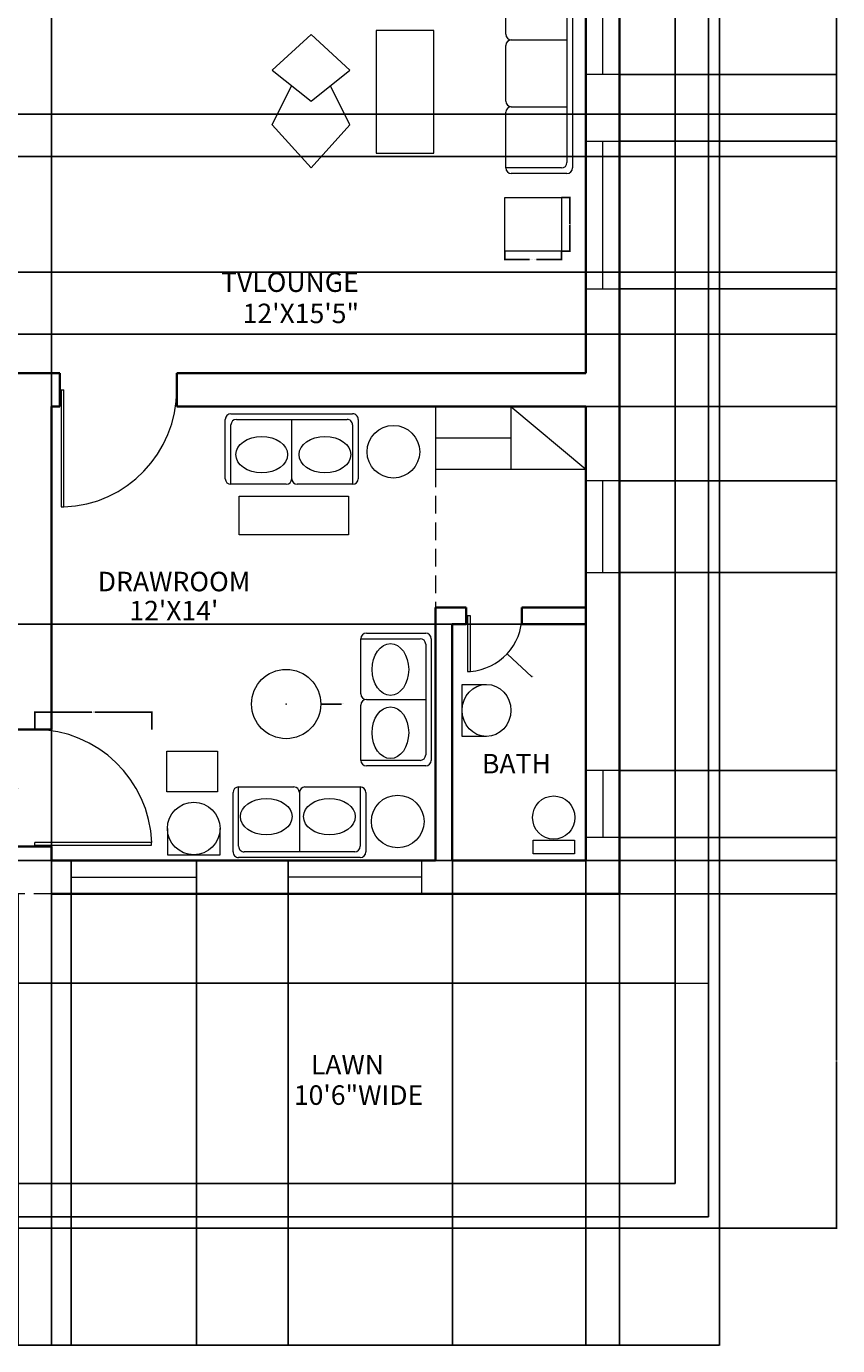
# Model space of a CAD drawing. Units: inches. Extents: x 2863 to 3499, y 1212 to 2136.
# Tile 4 of 7: x 3208 to 3499, y 1212 to 1686. Entities that reach past the tile are written whole.
import ezdxf

# ---------------------------------------------------------------- set-up
doc = ezdxf.new("R2010")
doc.units = ezdxf.units.IN
doc.linetypes.add('DASHED2', pattern=[9.525, 6.35, -3.175])
for name, color, linetype, lineweight in [('A-ANNO-DIMS', 2, 'Continuous', 18), ('A-AREA-IDEN', 7, 'Continuous', 18), ('A-DOOR', 221, 'Continuous', 18), ('A-FLOR-CASE', 254, 'Continuous', 18), ('A-FLOR-FIXT', 254, 'Continuous', 18), ('A-FLOR-OVHD', 51, 'DASHED2', 18), ('A-FURN', 131, 'Continuous', 18), ('A-GLAZ', 191, 'Continuous', 18), ('A-WALL', 51, 'Continuous', 35), ('C-PROP', 51, 'Continuous', 25), ('L-SITE-EDGE', 51, 'Continuous', 18)]:
    doc.layers.add(name, color=color, linetype=linetype, lineweight=lineweight)
doc.styles.get("Standard").update_dxf_attribs({"font": 'arial.ttf'})
doc.dimstyles.get("Standard").update_dxf_attribs({"dimtxt": 0.18, "dimasz": 0.18, "dimexe": 0.18, "dimexo": 0.0625, "dimgap": 0.09, "dimtad": 0, "dimtih": 1, "dimtoh": 1, "dimdec": 4, "dimzin": 0, "dimdsep": 46, "dimtxsty": 'Standard', "dimcen": 0.09, "dimadec": 0, "dimazin": 0, "dimtfac": 1, "dimtdec": 4, "dimtofl": 0, "dimtmove": 0, "dimatfit": 3, "dimfxl": 1, "dimtolj": 1, "dimtzin": 0, "dimarcsym": 0})

# ---------------------------------------------------------------- blocks, each defined once
blk = doc.blocks.new('SOFA-TWO-SEAT')
for p, q in [((2, 47.71), (23.32, 47.71)), ((0, 45.71), (21.32, 45.71)), ((0, 25.85), (0, 45.71)), ((23.32, 43.71), (23.32, 4)), ((25.32, 45.71), (25.32, 2)), ((2, 23.85), (23.32, 23.85)), ((2, 23.85), (2, 23.85)), ((0, 2), (0, 21.85)), ((21.32, 2), (0, 2)), ((23.32, 0), (2, 0))]:
    blk.add_line(p, q)
for centre, start, end in [((2, 45.71), 90, 180), ((23.32, 45.71), 0, 90), ((21.32, 43.71), 0, 90), ((2, 25.85), 180, 270), ((2, 21.85), 90, 180), ((2, 2), 180, 270), ((21.32, 4), 270, 0), ((23.32, 2), 270, 0)]:
    blk.add_arc(centre, 2, start, end)
for centre in [(10.66, 34.63), (10.66, 11.93)]:
    blk.add_ellipse(centre, major_axis=(0, 9.3), ratio=0.704902)
blk = doc.blocks.new('WC-CLOSE-COUPLED')
blk.add_lwpolyline([(0.19, 20.82), (15, 20.82), (15, 15.96), (0.19, 15.96)], close=True)
blk.add_ellipse((7.6, 7.79), major_axis=(0, 7.78), ratio=0.975839)
blk = doc.blocks.new('CHAIR-ROUND-BACK')
for p, q in [((18.9, 18.9), (0, 18.9)), ((0, 18.9), (0, 9.45)), ((18.9, 9.45), (18.9, 18.9))]:
    blk.add_line(p, q)
blk.add_circle((9.45, 9.45), 9.45)
blk = doc.blocks.new('TABLE-SIDE-ROUND')
blk.add_circle((9.45, 9.45), 9.45)
blk = doc.blocks.new('TABLE-SIDE-RECT')
blk.add_lwpolyline([(18.23, 14.69), (18.23, 0), (0, 0), (0, 14.69)], close=True)
blk = doc.blocks.new('TABLE-END-LOUNGE')
blk.add_lwpolyline([(0, 19.18), (20.36, 19.18), (20.36, 0), (0, 0)], close=True)
blk = doc.blocks.new('SOFA-THREE-SEAT')
for p, q in [((2, 24), (22, 24)), ((2, 4), (2, 24)), ((26, 24), (46, 24)), ((50, 24), (70, 24)), ((70, 24), (70, 4)), ((0, 2), (0, 22)), ((24, 22), (24, 2)), ((24, 22), (24, 22)), ((48, 22), (48, 2)), ((48, 22), (48, 22)), ((72, 22), (72, 2)), ((70, 0), (2, 0)), ((68, 2), (4, 2))]:
    blk.add_line(p, q)
for centre, start, end in [((2, 22), 90, 180), ((22, 22), 0, 90), ((26, 22), 90, 180), ((46, 22), 0, 90), ((50, 22), 90, 180), ((70, 22), 0, 90), ((2, 2), 180, 270), ((4, 4), 180, 270), ((68, 4), 270, 0), ((70, 2), 270, 0)]:
    blk.add_arc(centre, 2, start, end)
blk = doc.blocks.new('BASIN-WALL')
for p, q in [((8.77, 18.68), (17.53, 18.68)), ((17.53, 18.68), (17.53, 0)), ((17.53, 0), (8.77, 0))]:
    blk.add_line(p, q)
blk.add_ellipse((8.77, 9.34), major_axis=(0, 9.34), ratio=0.938307)
blk = doc.blocks.new('DOOR-SWING-42IN')
for p, q in [((42, 1.5), (0, 1.5)), ((0, 0.5), (0, 1.5)), ((0, 0), (0, 0.5)), ((0, 0.5), (42, 0.5)), ((42, 0.5), (42, 1.5))]:
    blk.add_line(p, q)
blk.add_arc((0.03, 0), 42, 2.0467, 90.0366)
blk = doc.blocks.new('WINDOW-24IN')
for p, q in [((12, 24), (0, 24)), ((6, 24), (6, 0)), ((12, 0), (0, 0))]:
    blk.add_line(p, q)
blk = doc.blocks.new('WINDOW-48IN')
for p, q in [((12, 48), (0, 48)), ((6, 48), (6, 0)), ((12, 0), (0, 0))]:
    blk.add_line(p, q)
blk = doc.blocks.new('WINDOW-56IN')
for p, q in [((12, 56), (0, 56)), ((6, 0), (6, 56)), ((12, 0), (0, 0))]:
    blk.add_line(p, q)
blk = doc.blocks.new('*D37')
at = {"layer": 'A-ANNO-DIMS', "color": 0, "lineweight": -2, "transparency": 16777216}
for p, q in [((3379.75, 1604.98), (3379.75, 1601.81)), ((3379.93, 1601.99), (3388.68, 1601.99)), ((3399.93, 1601.99), (3391.19, 1601.99)), ((3400.11, 1604.98), (3400.11, 1601.81))]:
    blk.add_line(p, q, dxfattribs=at)
at = {"layer": 'A-ANNO-DIMS', "color": 0, "transparency": 16777216}
for points in [[(3379.93, 1602.02), (3379.93, 1601.96), (3379.75, 1601.99)], [(3399.93, 1602.02), (3399.93, 1601.96), (3400.11, 1601.99)]]:
    blk.add_solid(points, dxfattribs=at)
at = {"layer": 'Defpoints', "color": 0, "transparency": 16777216}
for p in [(3379.75, 1605.04), (3400.11, 1605.04), (3400.11, 1601.99)]:
    blk.add_point(p, dxfattribs=at)
at = {"layer": 'A-ANNO-DIMS', "color": 0, "transparency": 16777216, "insert": (3389.93, 1601.99), "char_height": 0.18, "attachment_point": 5}
blk.add_mtext('\\A1;END TABLE 20 TYP.', dxfattribs=at)
blk = doc.blocks.new('*D38')
at = {"layer": 'A-ANNO-DIMS', "color": 0, "lineweight": -2, "transparency": 16777216}
for p, q in [((3400.18, 1624.22), (3403.35, 1624.22)), ((3403.17, 1624.04), (3403.17, 1614.81)), ((3403.17, 1605.22), (3403.17, 1614.45)), ((3400.18, 1605.04), (3403.35, 1605.04))]:
    blk.add_line(p, q, dxfattribs=at)
at = {"layer": 'A-ANNO-DIMS', "color": 0, "transparency": 16777216}
for points in [[(3403.14, 1624.04), (3403.2, 1624.04), (3403.17, 1624.22)], [(3403.14, 1605.22), (3403.2, 1605.22), (3403.17, 1605.04)]]:
    blk.add_solid(points, dxfattribs=at)
at = {"layer": 'Defpoints', "color": 0, "transparency": 16777216}
for p in [(3400.11, 1624.22), (3403.17, 1624.22), (3400.11, 1605.04)]:
    blk.add_point(p, dxfattribs=at)
at = {"layer": 'A-ANNO-DIMS', "color": 0, "transparency": 16777216, "insert": (3403.17, 1614.63), "char_height": 0.18, "attachment_point": 5}
blk.add_mtext('\\A1;19 TYP.', dxfattribs=at)
blk = doc.blocks.new('*D39')
at = {"layer": 'A-ANNO-DIMS', "color": 0, "lineweight": -2, "transparency": 16777216}
for p, q in [((3210.85, 1433.18), (3204.43, 1433.18)), ((3204.61, 1433), (3204.61, 1412.36)), ((3204.61, 1391.35), (3204.61, 1411.99)), ((3210.85, 1391.17), (3204.43, 1391.17))]:
    blk.add_line(p, q, dxfattribs=at)
at = {"layer": 'A-ANNO-DIMS', "color": 0, "transparency": 16777216}
for points in [[(3204.58, 1433), (3204.64, 1433), (3204.61, 1433.18)], [(3204.58, 1391.35), (3204.64, 1391.35), (3204.61, 1391.17)]]:
    blk.add_solid(points, dxfattribs=at)
at = {"layer": 'Defpoints', "color": 0, "transparency": 16777216}
for p in [(3204.61, 1433.18), (3210.92, 1433.18), (3210.92, 1391.17)]:
    blk.add_point(p, dxfattribs=at)
at = {"layer": 'A-ANNO-DIMS', "color": 0, "transparency": 16777216, "insert": (3204.61, 1412.17), "char_height": 0.18, "attachment_point": 5}
blk.add_mtext('\\A1;DOOR 42 TYP.', dxfattribs=at)
blk = doc.blocks.new('*D40')
at = {"layer": 'A-ANNO-DIMS', "color": 0, "lineweight": -2, "transparency": 16777216}
for p, q in [((3210.92, 1433.24), (3210.92, 1439.66)), ((3211.1, 1439.48), (3231.39, 1439.48)), ((3252.74, 1439.48), (3232.45, 1439.48)), ((3252.92, 1433.24), (3252.92, 1439.66))]:
    blk.add_line(p, q, dxfattribs=at)
at = {"layer": 'A-ANNO-DIMS', "color": 0, "transparency": 16777216}
for points in [[(3211.1, 1439.51), (3211.1, 1439.45), (3210.92, 1439.48)], [(3252.74, 1439.51), (3252.74, 1439.45), (3252.92, 1439.48)]]:
    blk.add_solid(points, dxfattribs=at)
at = {"layer": 'Defpoints', "color": 0, "transparency": 16777216}
for p in [(3252.92, 1439.48), (3210.92, 1433.18), (3252.92, 1433.18)]:
    blk.add_point(p, dxfattribs=at)
at = {"layer": 'A-ANNO-DIMS', "color": 0, "transparency": 16777216, "insert": (3231.92, 1439.48), "char_height": 0.18, "attachment_point": 5}
blk.add_mtext('\\A1;42 TYP.', dxfattribs=at)
blk = doc.blocks.new('*D49')
at = {"layer": 'A-ANNO-DIMS', "color": 0, "lineweight": -2, "transparency": 16777216}
for p, q in [((2904.92, 1254.1), (2904.92, 1211.97)), ((3456.92, 1254.1), (3456.92, 1211.97)), ((2905.1, 1212.15), (3180.63, 1212.15)), ((3456.74, 1212.15), (3181.2, 1212.15))]:
    blk.add_line(p, q, dxfattribs=at)
at = {"layer": 'A-ANNO-DIMS', "color": 0, "transparency": 16777216}
for points in [[(2905.1, 1212.18), (2905.1, 1212.12), (2904.92, 1212.15)], [(3456.74, 1212.18), (3456.74, 1212.12), (3456.92, 1212.15)]]:
    blk.add_solid(points, dxfattribs=at)
at = {"layer": 'Defpoints', "color": 0, "transparency": 16777216}
for p in [(2904.92, 1254.17), (3456.92, 1254.17), (3456.92, 1212.15)]:
    blk.add_point(p, dxfattribs=at)
at = {"layer": 'A-ANNO-DIMS', "color": 0, "transparency": 16777216, "insert": (3180.92, 1212.15), "char_height": 0.18, "attachment_point": 5}
blk.add_mtext('\\A1;552', dxfattribs=at)
blk = doc.blocks.new('*D57')
at = {"layer": 'A-ANNO-DIMS', "color": 0, "lineweight": -2, "transparency": 16777216}
for p, q in [((3456.98, 2094.17), (3499.12, 2094.17)), ((3498.94, 2093.99), (3498.94, 1734.35)), ((3498.94, 1374.35), (3498.94, 1733.98)), ((3452.98, 1374.17), (3499.12, 1374.17))]:
    blk.add_line(p, q, dxfattribs=at)
at = {"layer": 'A-ANNO-DIMS', "color": 0, "transparency": 16777216}
for points in [[(3498.91, 2093.99), (3498.97, 2093.99), (3498.94, 2094.17)], [(3498.91, 1374.35), (3498.97, 1374.35), (3498.94, 1374.17)]]:
    blk.add_solid(points, dxfattribs=at)
at = {"layer": 'Defpoints', "color": 0, "transparency": 16777216}
for p in [(3456.92, 2094.17), (3498.94, 2094.17), (3452.92, 1374.17)]:
    blk.add_point(p, dxfattribs=at)
at = {"layer": 'A-ANNO-DIMS', "color": 0, "transparency": 16777216, "insert": (3498.94, 1734.17), "char_height": 0.18, "attachment_point": 5}
blk.add_mtext('\\A1;720', dxfattribs=at)
blk = doc.blocks.new('*D58')
at = {"layer": 'A-ANNO-DIMS', "color": 0, "lineweight": -2, "transparency": 16777216}
for p, q in [((3452.98, 1374.17), (3499.12, 1374.17)), ((3498.94, 1373.99), (3498.94, 1314.35)), ((3498.94, 1254.35), (3498.94, 1313.98)), ((3456.98, 1254.17), (3499.12, 1254.17))]:
    blk.add_line(p, q, dxfattribs=at)
at = {"layer": 'A-ANNO-DIMS', "color": 0, "transparency": 16777216}
for points in [[(3498.91, 1373.99), (3498.97, 1373.99), (3498.94, 1374.17)], [(3498.91, 1254.35), (3498.97, 1254.35), (3498.94, 1254.17)]]:
    blk.add_solid(points, dxfattribs=at)
at = {"layer": 'Defpoints', "color": 0, "transparency": 16777216}
for p in [(3452.92, 1374.17), (3456.92, 1254.17), (3498.94, 1254.17)]:
    blk.add_point(p, dxfattribs=at)
at = {"layer": 'A-ANNO-DIMS', "color": 0, "transparency": 16777216, "insert": (3498.94, 1314.17), "char_height": 0.18, "attachment_point": 5}
blk.add_mtext('\\A1;120', dxfattribs=at)
blk = doc.blocks.new('*D59')
at = {"layer": 'A-ANNO-DIMS', "color": 0, "lineweight": -2, "transparency": 16777216}
for p, q in [((3408.98, 1549.17), (3499.12, 1549.17)), ((3498.94, 1548.99), (3498.94, 1467.85)), ((3498.94, 1386.35), (3498.94, 1467.48)), ((3408.98, 1386.17), (3499.12, 1386.17))]:
    blk.add_line(p, q, dxfattribs=at)
at = {"layer": 'A-ANNO-DIMS', "color": 0, "transparency": 16777216}
for points in [[(3498.91, 1548.99), (3498.97, 1548.99), (3498.94, 1549.17)], [(3498.91, 1386.35), (3498.97, 1386.35), (3498.94, 1386.17)]]:
    blk.add_solid(points, dxfattribs=at)
at = {"layer": 'Defpoints', "color": 0, "transparency": 16777216}
for p in [(3408.92, 1549.17), (3498.94, 1549.17), (3408.92, 1386.17)]:
    blk.add_point(p, dxfattribs=at)
at = {"layer": 'A-ANNO-DIMS', "color": 0, "transparency": 16777216, "insert": (3498.94, 1467.67), "char_height": 0.18, "attachment_point": 5}
blk.add_mtext('\\A1;163', dxfattribs=at)
blk = doc.blocks.new('*D60')
at = {"layer": 'A-ANNO-DIMS', "color": 0, "lineweight": -2, "transparency": 16777216}
for p, q in [((3408.98, 1746.17), (3499.12, 1746.17)), ((3498.94, 1745.99), (3498.94, 1647.85)), ((3498.94, 1549.35), (3498.94, 1647.48)), ((3408.98, 1549.17), (3499.12, 1549.17))]:
    blk.add_line(p, q, dxfattribs=at)
at = {"layer": 'A-ANNO-DIMS', "color": 0, "transparency": 16777216}
for points in [[(3498.91, 1745.99), (3498.97, 1745.99), (3498.94, 1746.17)], [(3498.91, 1549.35), (3498.97, 1549.35), (3498.94, 1549.17)]]:
    blk.add_solid(points, dxfattribs=at)
at = {"layer": 'Defpoints', "color": 0, "transparency": 16777216}
for p in [(3408.92, 1746.17), (3498.94, 1746.17), (3408.92, 1549.17)]:
    blk.add_point(p, dxfattribs=at)
at = {"layer": 'A-ANNO-DIMS', "color": 0, "transparency": 16777216, "insert": (3498.94, 1647.67), "char_height": 0.18, "attachment_point": 5}
blk.add_mtext('\\A1;197', dxfattribs=at)
blk = doc.blocks.new('*D71')
at = {"layer": 'A-ANNO-DIMS', "color": 0, "lineweight": -2, "transparency": 16777216}
for p, q in [((3204.92, 1374.1), (3204.92, 1211.97)), ((3420.92, 1374.1), (3420.92, 1211.97)), ((3205.1, 1212.15), (3312.63, 1212.15)), ((3420.74, 1212.15), (3313.21, 1212.15))]:
    blk.add_line(p, q, dxfattribs=at)
at = {"layer": 'A-ANNO-DIMS', "color": 0, "transparency": 16777216}
for points in [[(3205.1, 1212.18), (3205.1, 1212.12), (3204.92, 1212.15)], [(3420.74, 1212.18), (3420.74, 1212.12), (3420.92, 1212.15)]]:
    blk.add_solid(points, dxfattribs=at)
at = {"layer": 'Defpoints', "color": 0, "transparency": 16777216}
for p in [(3204.92, 1374.17), (3420.92, 1374.17), (3420.92, 1212.15)]:
    blk.add_point(p, dxfattribs=at)
at = {"layer": 'A-ANNO-DIMS', "color": 0, "transparency": 16777216, "insert": (3312.92, 1212.15), "char_height": 0.18, "attachment_point": 5}
blk.add_mtext('\\A1;216', dxfattribs=at)
blk = doc.blocks.new('*D73')
at = {"layer": 'A-ANNO-DIMS', "color": 0, "lineweight": -2, "transparency": 16777216}
for p, q in [((3360.92, 1386.1), (3360.92, 1211.97)), ((3408.92, 1386.1), (3408.92, 1211.97)), ((3361.1, 1212.15), (3384.69, 1212.15)), ((3408.74, 1212.15), (3385.14, 1212.15))]:
    blk.add_line(p, q, dxfattribs=at)
at = {"layer": 'A-ANNO-DIMS', "color": 0, "transparency": 16777216}
for points in [[(3361.1, 1212.18), (3361.1, 1212.12), (3360.92, 1212.15)], [(3408.74, 1212.18), (3408.74, 1212.12), (3408.92, 1212.15)]]:
    blk.add_solid(points, dxfattribs=at)
at = {"layer": 'Defpoints', "color": 0, "transparency": 16777216}
for p in [(3360.92, 1386.17), (3408.92, 1386.17), (3408.92, 1212.15)]:
    blk.add_point(p, dxfattribs=at)
at = {"layer": 'A-ANNO-DIMS', "color": 0, "transparency": 16777216, "insert": (3384.92, 1212.15), "char_height": 0.18, "attachment_point": 5}
blk.add_mtext('\\A1;48', dxfattribs=at)
blk = doc.blocks.new('*D74')
at = {"layer": 'A-ANNO-DIMS', "color": 0, "lineweight": -2, "transparency": 16777216}
for p, q in [((3408.85, 1471.09), (2862.72, 1471.09)), ((2862.9, 1470.91), (2862.9, 1428.81)), ((2862.9, 1386.35), (2862.9, 1428.44)), ((3408.85, 1386.17), (2862.72, 1386.17))]:
    blk.add_line(p, q, dxfattribs=at)
at = {"layer": 'A-ANNO-DIMS', "color": 0, "transparency": 16777216}
for points in [[(2862.87, 1470.91), (2862.93, 1470.91), (2862.9, 1471.09)], [(2862.87, 1386.35), (2862.93, 1386.35), (2862.9, 1386.17)]]:
    blk.add_solid(points, dxfattribs=at)
at = {"layer": 'Defpoints', "color": 0, "transparency": 16777216}
for p in [(3408.92, 1471.09), (2862.9, 1386.17), (3408.92, 1386.17)]:
    blk.add_point(p, dxfattribs=at)
at = {"layer": 'A-ANNO-DIMS', "color": 0, "transparency": 16777216, "insert": (2862.9, 1428.63), "char_height": 0.18, "attachment_point": 5}
blk.add_mtext('\\A1;84.92', dxfattribs=at)
blk = doc.blocks.new('*D80')
at = {"layer": 'A-ANNO-DIMS', "color": 0, "lineweight": -2, "transparency": 16777216}
for p, q in [((3081.48, 1638.96), (3499.12, 1638.96)), ((3498.94, 1638.78), (3498.94, 1618.41)), ((3498.94, 1597.68), (3498.94, 1618.05)), ((3081.48, 1597.5), (3499.12, 1597.5))]:
    blk.add_line(p, q, dxfattribs=at)
at = {"layer": 'A-ANNO-DIMS', "color": 0, "transparency": 16777216}
for points in [[(3498.91, 1638.78), (3498.97, 1638.78), (3498.94, 1638.96)], [(3498.91, 1597.68), (3498.97, 1597.68), (3498.94, 1597.5)]]:
    blk.add_solid(points, dxfattribs=at)
at = {"layer": 'Defpoints', "color": 0, "transparency": 16777216}
for p in [(3081.41, 1638.96), (3498.94, 1638.96), (3081.41, 1597.5)]:
    blk.add_point(p, dxfattribs=at)
at = {"layer": 'A-ANNO-DIMS', "color": 0, "transparency": 16777216, "insert": (3498.94, 1618.23), "char_height": 0.18, "attachment_point": 5}
blk.add_mtext('\\A1;41.46', dxfattribs=at)
blk = doc.blocks.new('*D82')
at = {"layer": 'A-ANNO-DIMS', "color": 0, "lineweight": -2, "transparency": 16777216}
for p, q in [((3121.98, 1654.17), (3499.12, 1654.17)), ((3498.94, 1653.99), (3498.94, 1614.85)), ((3498.94, 1575.35), (3498.94, 1614.48)), ((3121.98, 1575.17), (3499.12, 1575.17))]:
    blk.add_line(p, q, dxfattribs=at)
at = {"layer": 'A-ANNO-DIMS', "color": 0, "transparency": 16777216}
for points in [[(3498.91, 1653.99), (3498.97, 1653.99), (3498.94, 1654.17)], [(3498.91, 1575.35), (3498.97, 1575.35), (3498.94, 1575.17)]]:
    blk.add_solid(points, dxfattribs=at)
at = {"layer": 'Defpoints', "color": 0, "transparency": 16777216}
for p in [(3121.92, 1654.17), (3498.94, 1654.17), (3121.92, 1575.17)]:
    blk.add_point(p, dxfattribs=at)
at = {"layer": 'A-ANNO-DIMS', "color": 0, "transparency": 16777216, "insert": (3498.94, 1614.67), "char_height": 0.18, "attachment_point": 5}
blk.add_mtext('\\A1;79', dxfattribs=at)
blk = doc.blocks.new('*D90')
at = {"layer": 'A-ANNO-DIMS', "color": 0, "lineweight": -2, "transparency": 16777216}
for p, q in [((3420.98, 1394.44), (3499.12, 1394.44)), ((3498.94, 1394.26), (3498.94, 1384.49)), ((3498.94, 1374.35), (3498.94, 1384.12)), ((3420.98, 1374.17), (3499.12, 1374.17))]:
    blk.add_line(p, q, dxfattribs=at)
at = {"layer": 'A-ANNO-DIMS', "color": 0, "transparency": 16777216}
for points in [[(3498.91, 1394.26), (3498.97, 1394.26), (3498.94, 1394.44)], [(3498.91, 1374.35), (3498.97, 1374.35), (3498.94, 1374.17)]]:
    blk.add_solid(points, dxfattribs=at)
at = {"layer": 'Defpoints', "color": 0, "transparency": 16777216}
for p in [(3420.92, 1394.44), (3498.94, 1394.44), (3420.92, 1374.17)]:
    blk.add_point(p, dxfattribs=at)
at = {"layer": 'A-ANNO-DIMS', "color": 0, "transparency": 16777216, "insert": (3498.94, 1384.3), "char_height": 0.18, "attachment_point": 5}
blk.add_mtext('\\A1;20.28', dxfattribs=at)
blk = doc.blocks.new('*D91')
at = {"layer": 'A-ANNO-DIMS', "color": 0, "lineweight": -2, "transparency": 16777216}
for p, q in [((3420.98, 1489.58), (3499.12, 1489.58)), ((3498.94, 1489.4), (3498.94, 1454.19)), ((3498.94, 1418.62), (3498.94, 1453.83)), ((3420.98, 1418.44), (3499.12, 1418.44))]:
    blk.add_line(p, q, dxfattribs=at)
at = {"layer": 'A-ANNO-DIMS', "color": 0, "transparency": 16777216}
for points in [[(3498.91, 1489.4), (3498.97, 1489.4), (3498.94, 1489.58)], [(3498.91, 1418.62), (3498.97, 1418.62), (3498.94, 1418.44)]]:
    blk.add_solid(points, dxfattribs=at)
at = {"layer": 'Defpoints', "color": 0, "transparency": 16777216}
for p in [(3420.92, 1489.58), (3498.94, 1489.58), (3420.92, 1418.44)]:
    blk.add_point(p, dxfattribs=at)
at = {"layer": 'A-ANNO-DIMS', "color": 0, "transparency": 16777216, "insert": (3498.94, 1454.01), "char_height": 0.18, "attachment_point": 5}
blk.add_mtext('\\A1;71.14', dxfattribs=at)
blk = doc.blocks.new('*D92')
at = {"layer": 'A-ANNO-DIMS', "color": 0, "lineweight": -2, "transparency": 16777216}
for p, q in [((3420.98, 1522.58), (3499.12, 1522.58)), ((3498.94, 1522.4), (3498.94, 1506.26)), ((3498.94, 1489.76), (3498.94, 1505.9)), ((3420.98, 1489.58), (3499.12, 1489.58))]:
    blk.add_line(p, q, dxfattribs=at)
at = {"layer": 'A-ANNO-DIMS', "color": 0, "transparency": 16777216}
for points in [[(3498.91, 1522.4), (3498.97, 1522.4), (3498.94, 1522.58)], [(3498.91, 1489.76), (3498.97, 1489.76), (3498.94, 1489.58)]]:
    blk.add_solid(points, dxfattribs=at)
at = {"layer": 'Defpoints', "color": 0, "transparency": 16777216}
for p in [(3420.92, 1522.58), (3498.94, 1522.58), (3420.92, 1489.58)]:
    blk.add_point(p, dxfattribs=at)
at = {"layer": 'A-ANNO-DIMS', "color": 0, "transparency": 16777216, "insert": (3498.94, 1506.08), "char_height": 0.18, "attachment_point": 5}
blk.add_mtext('\\A1;33', dxfattribs=at)
blk = doc.blocks.new('*D93')
at = {"layer": 'A-ANNO-DIMS', "color": 0, "lineweight": -2, "transparency": 16777216}
for p, q in [((3420.98, 1591.45), (3499.12, 1591.45)), ((3498.94, 1591.27), (3498.94, 1557.2)), ((3498.94, 1522.76), (3498.94, 1556.83)), ((3420.98, 1522.58), (3499.12, 1522.58))]:
    blk.add_line(p, q, dxfattribs=at)
at = {"layer": 'A-ANNO-DIMS', "color": 0, "transparency": 16777216}
for points in [[(3498.91, 1591.27), (3498.97, 1591.27), (3498.94, 1591.45)], [(3498.91, 1522.76), (3498.97, 1522.76), (3498.94, 1522.58)]]:
    blk.add_solid(points, dxfattribs=at)
at = {"layer": 'Defpoints', "color": 0, "transparency": 16777216}
for p in [(3420.92, 1591.45), (3498.94, 1591.45), (3420.92, 1522.58)]:
    blk.add_point(p, dxfattribs=at)
at = {"layer": 'A-ANNO-DIMS', "color": 0, "transparency": 16777216, "insert": (3498.94, 1557.01), "char_height": 0.18, "attachment_point": 5}
blk.add_mtext('\\A1;68.86', dxfattribs=at)
blk = doc.blocks.new('*D94')
at = {"layer": 'A-ANNO-DIMS', "color": 0, "lineweight": -2, "transparency": 16777216}
for p, q in [((3420.98, 1644.45), (3499.12, 1644.45)), ((3498.94, 1644.27), (3498.94, 1618.13)), ((3498.94, 1591.63), (3498.94, 1617.76)), ((3420.98, 1591.45), (3499.12, 1591.45))]:
    blk.add_line(p, q, dxfattribs=at)
at = {"layer": 'A-ANNO-DIMS', "color": 0, "transparency": 16777216}
for points in [[(3498.91, 1644.27), (3498.97, 1644.27), (3498.94, 1644.45)], [(3498.91, 1591.63), (3498.97, 1591.63), (3498.94, 1591.45)]]:
    blk.add_solid(points, dxfattribs=at)
at = {"layer": 'Defpoints', "color": 0, "transparency": 16777216}
for p in [(3420.92, 1644.45), (3498.94, 1644.45), (3420.92, 1591.45)]:
    blk.add_point(p, dxfattribs=at)
at = {"layer": 'A-ANNO-DIMS', "color": 0, "transparency": 16777216, "insert": (3498.94, 1617.95), "char_height": 0.18, "attachment_point": 5}
blk.add_mtext('\\A1;53', dxfattribs=at)
blk = doc.blocks.new('*D95')
at = {"layer": 'A-ANNO-DIMS', "color": 0, "lineweight": -2, "transparency": 16777216}
for p, q in [((3420.98, 1668.49), (3499.12, 1668.49)), ((3498.94, 1668.31), (3498.94, 1656.65)), ((3498.94, 1644.63), (3498.94, 1656.29)), ((3420.98, 1644.45), (3499.12, 1644.45))]:
    blk.add_line(p, q, dxfattribs=at)
at = {"layer": 'A-ANNO-DIMS', "color": 0, "transparency": 16777216}
for points in [[(3498.91, 1668.31), (3498.97, 1668.31), (3498.94, 1668.49)], [(3498.91, 1644.63), (3498.97, 1644.63), (3498.94, 1644.45)]]:
    blk.add_solid(points, dxfattribs=at)
at = {"layer": 'Defpoints', "color": 0, "transparency": 16777216}
for p in [(3420.92, 1668.49), (3498.94, 1668.49), (3420.92, 1644.45)]:
    blk.add_point(p, dxfattribs=at)
at = {"layer": 'A-ANNO-DIMS', "color": 0, "transparency": 16777216, "insert": (3498.94, 1656.47), "char_height": 0.18, "attachment_point": 5}
blk.add_mtext('\\A1;24.047', dxfattribs=at)
blk = doc.blocks.new('*D104')
at = {"layer": 'A-ANNO-DIMS', "color": 0, "lineweight": -2, "transparency": 16777216}
for p, q in [((3216.92, 1386.1), (3216.92, 1211.97)), ((3223.99, 1386.1), (3223.99, 1211.97)), ((3217.1, 1212.15), (3220.08, 1212.15)), ((3223.81, 1212.15), (3220.83, 1212.15))]:
    blk.add_line(p, q, dxfattribs=at)
at = {"layer": 'A-ANNO-DIMS', "color": 0, "transparency": 16777216}
for points in [[(3217.1, 1212.18), (3217.1, 1212.12), (3216.92, 1212.15)], [(3223.81, 1212.18), (3223.81, 1212.12), (3223.99, 1212.15)]]:
    blk.add_solid(points, dxfattribs=at)
at = {"layer": 'Defpoints', "color": 0, "transparency": 16777216}
for p in [(3216.92, 1386.17), (3223.99, 1386.17), (3223.99, 1212.15)]:
    blk.add_point(p, dxfattribs=at)
at = {"layer": 'A-ANNO-DIMS', "color": 0, "transparency": 16777216, "insert": (3220.45, 1212.15), "char_height": 0.18, "attachment_point": 5}
blk.add_mtext('\\A1;7.071', dxfattribs=at)
blk = doc.blocks.new('*D105')
at = {"layer": 'A-ANNO-DIMS', "color": 0, "lineweight": -2, "transparency": 16777216}
for p, q in [((3223.99, 1386.1), (3223.99, 1211.97)), ((3268.99, 1386.1), (3268.99, 1211.97)), ((3224.17, 1212.15), (3246.26, 1212.15)), ((3268.81, 1212.15), (3246.71, 1212.15))]:
    blk.add_line(p, q, dxfattribs=at)
at = {"layer": 'A-ANNO-DIMS', "color": 0, "transparency": 16777216}
for points in [[(3224.17, 1212.18), (3224.17, 1212.12), (3223.99, 1212.15)], [(3268.81, 1212.18), (3268.81, 1212.12), (3268.99, 1212.15)]]:
    blk.add_solid(points, dxfattribs=at)
at = {"layer": 'Defpoints', "color": 0, "transparency": 16777216}
for p in [(3223.99, 1386.17), (3268.99, 1386.17), (3268.99, 1212.15)]:
    blk.add_point(p, dxfattribs=at)
at = {"layer": 'A-ANNO-DIMS', "color": 0, "transparency": 16777216, "insert": (3246.49, 1212.15), "char_height": 0.18, "attachment_point": 5}
blk.add_mtext('\\A1;45', dxfattribs=at)
blk = doc.blocks.new('*D106')
at = {"layer": 'A-ANNO-DIMS', "color": 0, "lineweight": -2, "transparency": 16777216}
for p, q in [((3268.99, 1386.1), (3268.99, 1211.97)), ((3301.94, 1386.1), (3301.94, 1211.97)), ((3269.17, 1212.15), (3285, 1212.15)), ((3301.76, 1212.15), (3285.93, 1212.15))]:
    blk.add_line(p, q, dxfattribs=at)
at = {"layer": 'A-ANNO-DIMS', "color": 0, "transparency": 16777216}
for points in [[(3269.17, 1212.18), (3269.17, 1212.12), (3268.99, 1212.15)], [(3301.76, 1212.18), (3301.76, 1212.12), (3301.94, 1212.15)]]:
    blk.add_solid(points, dxfattribs=at)
at = {"layer": 'Defpoints', "color": 0, "transparency": 16777216}
for p in [(3268.99, 1386.17), (3301.94, 1386.17), (3301.94, 1212.15)]:
    blk.add_point(p, dxfattribs=at)
at = {"layer": 'A-ANNO-DIMS', "color": 0, "transparency": 16777216, "insert": (3285.46, 1212.15), "char_height": 0.18, "attachment_point": 5}
blk.add_mtext('\\A1;32.954', dxfattribs=at)
blk = doc.blocks.new('*D107')
at = {"layer": 'A-ANNO-DIMS', "color": 0, "lineweight": -2, "transparency": 16777216}
for p, q in [((3216.92, 1270.23), (3216.92, 2136.37)), ((3217.1, 2136.19), (3328.63, 2136.19)), ((3440.74, 2136.19), (3329.21, 2136.19)), ((3440.92, 1270.23), (3440.92, 2136.37))]:
    blk.add_line(p, q, dxfattribs=at)
at = {"layer": 'A-ANNO-DIMS', "color": 0, "transparency": 16777216}
for points in [[(3217.1, 2136.22), (3217.1, 2136.16), (3216.92, 2136.19)], [(3440.74, 2136.22), (3440.74, 2136.16), (3440.92, 2136.19)]]:
    blk.add_solid(points, dxfattribs=at)
at = {"layer": 'Defpoints', "color": 0, "transparency": 16777216}
for p in [(3440.92, 2136.19), (3216.92, 1270.17), (3440.92, 1270.17)]:
    blk.add_point(p, dxfattribs=at)
at = {"layer": 'A-ANNO-DIMS', "color": 0, "transparency": 16777216, "insert": (3328.92, 2136.19), "char_height": 0.18, "attachment_point": 5}
blk.add_mtext('\\A1;224', dxfattribs=at)
blk = doc.blocks.new('*D108')
at = {"layer": 'A-ANNO-DIMS', "color": 0, "lineweight": -2, "transparency": 16777216}
for p, q in [((3440.85, 1342.09), (2862.72, 1342.09)), ((2862.9, 1341.91), (2862.9, 1306.31)), ((2862.9, 1270.35), (2862.9, 1305.95)), ((3440.85, 1270.17), (2862.72, 1270.17))]:
    blk.add_line(p, q, dxfattribs=at)
at = {"layer": 'A-ANNO-DIMS', "color": 0, "transparency": 16777216}
for points in [[(2862.87, 1341.91), (2862.93, 1341.91), (2862.9, 1342.09)], [(2862.87, 1270.35), (2862.93, 1270.35), (2862.9, 1270.17)]]:
    blk.add_solid(points, dxfattribs=at)
at = {"layer": 'Defpoints', "color": 0, "transparency": 16777216}
for p in [(2862.9, 1342.09), (3440.92, 1342.09), (3440.92, 1270.17)]:
    blk.add_point(p, dxfattribs=at)
at = {"layer": 'A-ANNO-DIMS', "color": 0, "transparency": 16777216, "insert": (2862.9, 1306.13), "char_height": 0.18, "attachment_point": 5}
blk.add_mtext('\\A1;71.93', dxfattribs=at)
blk = doc.blocks.new('*D118')
at = {"layer": 'A-ANNO-DIMS', "color": 0, "lineweight": -2, "transparency": 16777216}
for p, q in [((3365.83, 1474.03), (3366.01, 1474.03)), ((3365.92, 1473.94), (3365.92, 1474.12)), ((3389.41, 1452.3), (3380.73, 1460.33)), ((3389.59, 1452.3), (3389.41, 1452.3))]:
    blk.add_line(p, q, dxfattribs=at)
at = {"layer": 'A-ANNO-DIMS', "color": 0, "transparency": 16777216}
blk.add_solid([(3380.75, 1460.35), (3380.71, 1460.31), (3380.6, 1460.45)], dxfattribs=at)
at = {"layer": 'Defpoints', "color": 0, "transparency": 16777216}
for p in [(3365.92, 1474.03), (3380.6, 1460.45)]:
    blk.add_point(p, dxfattribs=at)
at = {"layer": 'A-ANNO-DIMS', "color": 0, "transparency": 16777216, "insert": (3389.89, 1452.3), "char_height": 0.18, "attachment_point": 5}
blk.add_mtext('\\A1;R20', dxfattribs=at)
blk = doc.blocks.new('*D120')
at = {"layer": 'A-ANNO-DIMS', "color": 0, "lineweight": -2, "transparency": 16777216}
for p, q in [((3301.14, 1442.37), (3301.32, 1442.37)), ((3301.23, 1442.28), (3301.23, 1442.46)), ((3321.14, 1442.37), (3313.85, 1442.37))]:
    blk.add_line(p, q, dxfattribs=at)
at = {"layer": 'A-ANNO-DIMS', "color": 0, "transparency": 16777216}
blk.add_solid([(3313.85, 1442.4), (3313.85, 1442.34), (3313.67, 1442.37)], dxfattribs=at)
at = {"layer": 'Defpoints', "color": 0, "transparency": 16777216}
for p in [(3288.78, 1442.37), (3313.67, 1442.37)]:
    blk.add_point(p, dxfattribs=at)
at = {"layer": 'A-ANNO-DIMS', "color": 0, "transparency": 16777216, "insert": (3321.63, 1442.37), "char_height": 0.18, "attachment_point": 5}
blk.add_mtext('\\A1;∅24.89', dxfattribs=at)

msp = doc.modelspace()

# ---------------------------------------------------------------- linework, layer by layer
at = {"layer": 'A-DOOR'}
for p, q in [((3365.9168, 1474.0882), (3366.4168, 1474.0882)), ((3366.4168, 1474.0882), (3366.4168, 1454.0882)), ((3367.4168, 1474.0882), (3366.4168, 1474.0882)), ((3367.4168, 1454.0882), (3367.4168, 1474.0882)), ((3366.4168, 1454.0882), (3367.4168, 1454.0882))]:
    msp.add_line(p, q, dxfattribs=at)
msp.add_arc((3365.9168, 1474.0318), 20, 274.300994, 0.161355, dxfattribs=at)
at = {"layer": 'A-FLOR-CASE'}
for p, q in [((3381.9168, 1549.1651), (3381.9168, 1526.6571)), ((3381.9168, 1549.1651), (3408.9168, 1526.6571)), ((3354.9168, 1537.9111), (3381.9168, 1537.9111))]:
    msp.add_line(p, q, dxfattribs=at)
msp.add_lwpolyline([(3408.9168, 1549.1651), (3354.9168, 1549.1651), (3354.9168, 1526.6571), (3408.9168, 1526.6571)], close=True, dxfattribs=at)
at = {"layer": 'A-FLOR-OVHD'}
for p, q in [((3354.9168, 1526.6571), (3354.9168, 1477.0882)), ((3216.9168, 1374.1651), (2940.9168, 1374.1651))]:
    msp.add_line(p, q, dxfattribs=at)
at = {"layer": 'A-FURN'}
for p, q in [((3296.2183, 1669.9728), (3310.1597, 1682.7728)), ((3310.1597, 1682.7728), (3324.1011, 1669.9728)), ((3296.2183, 1669.9728), (3310.1597, 1658.8669)), ((3310.1597, 1658.8669), (3324.1011, 1669.9728)), ((3296.2183, 1650.3963), (3303.189, 1664.4198)), ((3324.1011, 1650.3963), (3317.1304, 1664.4198)), ((3310.1597, 1634.961), (3296.2183, 1650.3963)), ((3324.1011, 1650.3963), (3310.1597, 1634.961))]:
    msp.add_line(p, q, dxfattribs=at)
for points in [[(3354.2447, 1684.2787), (3333.521, 1684.2787), (3333.521, 1640.2316), (3354.2447, 1640.2316)], [(3284.3934, 1517.0627), (3323.6713, 1517.0627), (3323.6713, 1503.1023), (3284.3934, 1503.1023)]]:
    msp.add_lwpolyline(points, close=True, dxfattribs=at)
msp.add_circle((3301.2277, 1442.367), 12.4447, dxfattribs=at)
at = {"layer": 'A-GLAZ'}
for p, q in [((3408.9168, 1644.4464), (3420.9168, 1644.4464)), ((3414.9168, 1644.4464), (3414.9168, 1591.4464)), ((3408.9168, 1591.4464), (3420.9168, 1591.4464)), ((3408.9168, 1522.5828), (3420.9168, 1522.5828)), ((3414.9168, 1522.5828), (3414.9168, 1489.5828)), ((3408.9168, 1489.5828), (3420.9168, 1489.5828)), ((3223.9877, 1386.1651), (3223.9877, 1374.1651)), ((3268.9877, 1386.1651), (3268.9877, 1374.1651)), ((3223.9877, 1380.1651), (3268.9877, 1380.1651))]:
    msp.add_line(p, q, dxfattribs=at)
at = {"layer": 'A-WALL'}
for p, q in [((3408.9168, 1926.1651), (3408.9168, 1561.1651)), ((3204.9168, 1561.1651), (3219.9168, 1561.1651)), ((3204.9168, 1561.1651), (3219.9168, 1561.1651)), ((3219.9168, 1561.1651), (3219.9168, 1549.1651)), ((3261.9168, 1561.1651), (3261.9168, 1549.1651)), ((3261.9168, 1561.1651), (3408.9168, 1561.1651)), ((3216.9168, 1549.1651), (3216.9168, 1433.1651)), ((3216.9168, 1549.1651), (3219.9168, 1549.1651)), ((3261.9168, 1549.1651), (3408.9168, 1549.1651)), ((3408.9168, 1549.1651), (3408.9168, 1386.1651)), ((3354.9168, 1477.0882), (3354.9168, 1386.1651)), ((3354.9168, 1477.0882), (3365.9168, 1477.0882)), ((3365.9168, 1471.0882), (3365.9168, 1477.0882)), ((3385.9168, 1471.0882), (3385.9168, 1477.0882)), ((3385.9168, 1477.0882), (3408.9168, 1477.0882)), ((3360.9168, 1471.0882), (3360.9168, 1386.1651)), ((3360.9168, 1471.0882), (3365.9168, 1471.0882)), ((3360.9168, 1471.0882), (3365.9168, 1471.0882)), ((3385.9168, 1471.0882), (3408.9168, 1471.0882)), ((3204.9168, 1433.1651), (3216.9168, 1433.1651)), ((3204.9168, 1391.1651), (3216.9168, 1391.1651)), ((3216.9168, 1391.1651), (3216.9168, 1386.1651)), ((3354.9168, 1386.1651), (3216.9168, 1386.1651)), ((3408.9168, 1386.1651), (3360.9168, 1386.1651))]:
    msp.add_line(p, q, dxfattribs=at)
msp.add_lwpolyline([(2940.9168, 1453.1651), (2940.9168, 2094.1651), (3420.9168, 2094.1651), (3420.9168, 1374.1651), (3216.9168, 1374.1651)], dxfattribs=at)
at = {"layer": 'C-PROP'}
for p, q in [((3452.9168, 1258.1651), (3452.9168, 2094.1651)), ((3456.9168, 2094.1651), (3456.9168, 1254.1651)), ((2908.9168, 1258.1651), (3452.9168, 1258.1651)), ((3456.9168, 1254.1651), (2904.9168, 1254.1651))]:
    msp.add_line(p, q, dxfattribs=at)
at = {"layer": 'L-SITE-EDGE'}
for p, q in [((3216.9168, 1386.1651), (3216.9168, 1258.1651)), ((3420.9168, 1374.1651), (3452.9168, 1374.1651)), ((3440.9168, 1270.1651), (3440.9168, 1342.0939)), ((3440.9168, 1342.0939), (3452.9168, 1342.0939)), ((3216.9168, 1270.1651), (3440.9168, 1270.1651))]:
    msp.add_line(p, q, dxfattribs=at)

# ---------------------------------------------------------------- block references
at = {"layer": 'A-DOOR', "rotation": 269.999999999998}
msp.add_blockref('DOOR-SWING-42IN', (3219.9167, 1555.1648), dxfattribs=at)
at = {"layer": 'A-DOOR'}
msp.add_blockref('DOOR-SWING-42IN', (3210.917, 1391.165), dxfattribs=at)
at = {"layer": 'A-FLOR-FIXT', "rotation": 180}
for name, p in [('BASIN-WALL', (3381.955, 1449.4218)), ('WC-CLOSE-COUPLED', (3404.937, 1409.3811))]:
    msp.add_blockref(name, p, dxfattribs=at)
at = {"layer": 'A-FURN'}
for name, p, rotation in [('SOFA-THREE-SEAT', (3404.1005, 1632.8692), 89.99999999999898), ('SOFA-TWO-SEAT', (3327.0896, 1521.2767), 89.99999999999967), ('TABLE-SIDE-RECT', (3276.5874, 1425.481), 180), ('SOFA-TWO-SEAT', (3282.1428, 1412.5861), 269.9999999999976), ('CHAIR-ROUND-BACK', (3277.4764, 1407.116), 180)]:
    msp.add_blockref(name, p, dxfattribs=dict(at, rotation=rotation))
for name, p in [('TABLE-END-LOUNGE', (3379.75, 1605.0428)), ('TABLE-SIDE-ROUND', (3330.2954, 1523.5203)), ('SOFA-TWO-SEAT', (3328.0307, 1420.1315)), ('TABLE-SIDE-ROUND', (3331.8426, 1390.7384))]:
    msp.add_blockref(name, p, dxfattribs=at)
at = {"layer": 'A-GLAZ'}
for name, p in [('WINDOW-56IN', (3408.917, 1668.4939)), ('WINDOW-24IN', (3408.917, 1394.4445))]:
    msp.add_blockref(name, p, dxfattribs=at)
at = {"layer": 'A-GLAZ', "rotation": 269.9999999999994}
msp.add_blockref('WINDOW-48IN', (3301.9416, 1386.1648), dxfattribs=at)

# ---------------------------------------------------------------- texts
at = {"layer": 'A-AREA-IDEN'}
for tag, p in [('TVLOUNGE', (3277.8354, 1590.3677)), ('12\'X15\'5"', (3285.6043, 1579.1473)), ('DRAWROOM', (3233.561, 1482.8552)), ("12'X14'", (3244.894, 1472.4259)), ('BATH', (3371.5583, 1417.4423)), ('LAWN', (3310.0986, 1309.3558)), ('10\'6"WIDE', (3303.9963, 1298.431))]:
    msp.add_attdef(tag, p, '', height=7, dxfattribs=at)

# ---------------------------------------------------------------- dimensions: what is measured, and where the dimension line sits
at = {"layer": 'A-ANNO-DIMS'}
for base, p1, p2, override, picture, middle in [((3440.9168, 2136.1851), (3216.9168, 1270.1651), (3440.9168, 1270.1651), {"dimdec": 0, "dimlfac": 1, "dimrnd": 0, "dimzin": 0, "dimdsep": 46, "dimlunit": 2}, '*D107', (3328.9168, 2136.1851)), ((3223.9877, 1212.1451), (3216.9168, 1386.1651), (3223.9877, 1386.1651), {"dimdec": 3, "dimlfac": 1, "dimrnd": 0, "dimzin": 0, "dimdsep": 46, "dimlunit": 2}, '*D104', (3220.4522, 1212.1451)), ((3268.9877, 1212.1451), (3223.9877, 1386.1651), (3268.9877, 1386.1651), {"dimdec": 0, "dimlfac": 1, "dimrnd": 0, "dimzin": 0, "dimdsep": 46, "dimlunit": 2}, '*D105', (3246.4877, 1212.1451)), ((3301.9416, 1212.1451), (3268.9877, 1386.1651), (3301.9416, 1386.1651), {"dimdec": 3, "dimlfac": 1, "dimrnd": 0, "dimzin": 0, "dimdsep": 46, "dimlunit": 2}, '*D106', (3285.4647, 1212.1451)), ((3408.9168, 1212.1451), (3360.9168, 1386.1651), (3408.9168, 1386.1651), {"dimdec": 0, "dimlfac": 1, "dimrnd": 0, "dimzin": 0, "dimdsep": 46, "dimlunit": 2}, '*D73', (3384.9168, 1212.1451)), ((3420.9168, 1212.1451), (3204.9168, 1374.1651), (3420.9168, 1374.1651), {"dimdec": 0, "dimlfac": 1, "dimrnd": 0, "dimzin": 0, "dimdsep": 46, "dimlunit": 2}, '*D71', (3312.9168, 1212.1451)), ((3456.9168, 1212.1451), (2904.9168, 1254.1651), (3456.9168, 1254.1651), {"dimdec": 0, "dimlfac": 1, "dimrnd": 0, "dimzin": 0, "dimdsep": 46, "dimlunit": 2}, '*D49', (3180.9168, 1212.1451))]:
    dim = msp.add_linear_dim(base=base, p1=p1, p2=p2, dimstyle='Standard', override=override, dxfattribs=at)
    dim.commit()
    dim.dimension.update_dxf_attribs({"geometry": picture, "text_midpoint": middle})
for base, p1, p2, override, picture, middle in [((3498.9368, 2094.1651), (3452.9168, 1374.1651), (3456.9168, 2094.1651), {"dimdec": 0, "dimlfac": 1, "dimrnd": 0, "dimzin": 0, "dimdsep": 46, "dimlunit": 2}, '*D57', (3498.9368, 1734.1651)), ((3498.9368, 1746.1651), (3408.9168, 1549.1651), (3408.9168, 1746.1651), {"dimdec": 0, "dimlfac": 1, "dimrnd": 0, "dimzin": 0, "dimdsep": 46, "dimlunit": 2}, '*D60', (3498.9368, 1647.6651)), ((3498.9368, 1668.4934), (3420.9168, 1644.4464), (3420.9168, 1668.4934), {"dimdec": 3, "dimlfac": 1, "dimrnd": 0, "dimzin": 0, "dimdsep": 46, "dimlunit": 2}, '*D95', (3498.9368, 1656.4699)), ((3498.9368, 1654.1651), (3121.9168, 1575.1651), (3121.9168, 1654.1651), {"dimdec": 0, "dimlfac": 1, "dimrnd": 0, "dimzin": 0, "dimdsep": 46, "dimlunit": 2}, '*D82', (3498.9368, 1614.6651)), ((3498.9368, 1644.4464), (3420.9168, 1591.4464), (3420.9168, 1644.4464), {"dimdec": 0, "dimlfac": 1, "dimrnd": 0, "dimzin": 0, "dimdsep": 46, "dimlunit": 2}, '*D94', (3498.9368, 1617.9464)), ((3498.9368, 1638.9588), (3081.415, 1597.4979), (3081.415, 1638.9588), {"dimdec": 2, "dimlfac": 1, "dimrnd": 0, "dimzin": 0, "dimdsep": 46, "dimlunit": 2}, '*D80', (3498.9368, 1618.2284)), ((3498.9368, 1591.4464), (3420.9168, 1522.5828), (3420.9168, 1591.4464), {"dimdec": 2, "dimlfac": 1, "dimrnd": 0, "dimzin": 0, "dimdsep": 46, "dimlunit": 2}, '*D93', (3498.9368, 1557.0146)), ((3498.9368, 1549.1651), (3408.9168, 1386.1651), (3408.9168, 1549.1651), {"dimdec": 0, "dimlfac": 1, "dimrnd": 0, "dimzin": 0, "dimdsep": 46, "dimlunit": 2}, '*D59', (3498.9368, 1467.6651)), ((3498.9368, 1522.5828), (3420.9168, 1489.5828), (3420.9168, 1522.5828), {"dimdec": 0, "dimlfac": 1, "dimrnd": 0, "dimzin": 0, "dimdsep": 46, "dimlunit": 2}, '*D92', (3498.9368, 1506.0828)), ((3498.9368, 1489.5828), (3420.9168, 1418.444), (3420.9168, 1489.5828), {"dimdec": 2, "dimlfac": 1, "dimrnd": 0, "dimzin": 0, "dimdsep": 46, "dimlunit": 2}, '*D91', (3498.9368, 1454.0134)), ((2862.8968, 1386.1651), (3408.9168, 1471.0882), (3408.9168, 1386.1651), {"dimdec": 2, "dimlfac": 1, "dimrnd": 0, "dimzin": 0, "dimdsep": 46, "dimlunit": 2}, '*D74', (2862.8968, 1428.6266)), ((3498.9368, 1394.444), (3420.9168, 1374.1651), (3420.9168, 1394.444), {"dimdec": 2, "dimlfac": 1, "dimrnd": 0, "dimzin": 0, "dimdsep": 46, "dimlunit": 2}, '*D90', (3498.9368, 1384.3046)), ((3498.9368, 1254.1651), (3452.9168, 1374.1651), (3456.9168, 1254.1651), {"dimdec": 0, "dimlfac": 1, "dimrnd": 0, "dimzin": 0, "dimdsep": 46, "dimlunit": 2}, '*D58', (3498.9368, 1314.1651)), ((2862.8968, 1342.0939), (3440.9168, 1270.1651), (3440.9168, 1342.0939), {"dimdec": 2, "dimlfac": 1, "dimrnd": 0, "dimzin": 0, "dimdsep": 46, "dimlunit": 2}, '*D108', (2862.8968, 1306.1295))]:
    dim = msp.add_linear_dim(base=base, p1=p1, p2=p2, angle=90, dimstyle='Standard', override=override, dxfattribs=at)
    dim.commit()
    dim.dimension.update_dxf_attribs({"geometry": picture, "text_midpoint": middle})
for base, p1, p2, text, picture, middle in [((3403.1697, 1624.2206), (3400.1149, 1605.0425), (3400.1149, 1624.2206), '<> TYP.', '*D38', (3403.1697, 1614.6315)), ((3204.6146, 1433.1795), (3210.9168, 1391.1651), (3210.9168, 1433.1795), 'DOOR <> TYP.', '*D39', (3204.6146, 1412.1723))]:
    dim = msp.add_linear_dim(base=base, p1=p1, p2=p2, angle=90, text=text, dimstyle='Standard', override={"dimdec": 0, "dimlfac": 1, "dimrnd": 0, "dimzin": 0, "dimdsep": 46, "dimlunit": 2}, dxfattribs=at)
    dim.commit()
    dim.dimension.update_dxf_attribs({"geometry": picture, "text_midpoint": middle})
for base, p1, p2, text, picture, middle in [((3400.1149, 1601.9877), (3379.7499, 1605.0425), (3400.1149, 1605.0425), 'END TABLE <> TYP.', '*D37', (3389.9324, 1601.9877)), ((3252.9168, 1439.4817), (3210.9168, 1433.1795), (3252.9168, 1433.1795), '<> TYP.', '*D40', (3231.9168, 1439.4817))]:
    dim = msp.add_linear_dim(base=base, p1=p1, p2=p2, text=text, dimstyle='Standard', override={"dimdec": 0, "dimlfac": 1, "dimrnd": 0, "dimzin": 0, "dimdsep": 46, "dimlunit": 2}, dxfattribs=at)
    dim.commit()
    dim.dimension.update_dxf_attribs({"geometry": picture, "text_midpoint": middle})
dim = msp.add_radius_dim(center=(3365.9168, 1474.0318), mpoint=(3380.5989, 1460.4511), dimstyle='Standard', override={"dimdec": 0, "dimlfac": 1, "dimrnd": 0, "dimzin": 0, "dimdsep": 46, "dimlunit": 2}, dxfattribs=at)
dim.commit()
dim.dimension.update_dxf_attribs({"geometry": '*D118', "text_midpoint": (3389.8929, 1452.3026), "dimtype": 164})
dim = msp.add_diameter_dim_2p(p1=(3288.783, 1442.367), p2=(3313.6724, 1442.367), dimstyle='Standard', override={"dimdec": 2, "dimlfac": 1, "dimrnd": 0, "dimzin": 0, "dimdsep": 46, "dimlunit": 2}, dxfattribs=at)
dim.commit()
dim.dimension.update_dxf_attribs({"geometry": '*D120', "text_midpoint": (3321.1393, 1442.367), "dimtype": 163})

doc.saveas('drawing.dxf')
